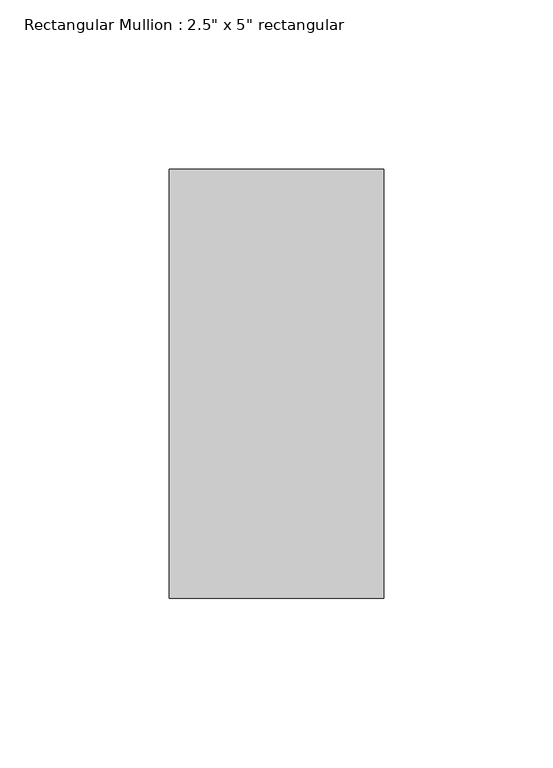
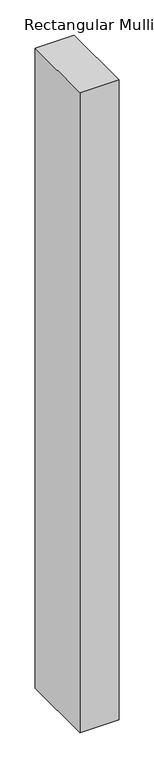
"""IFC4 building model written with IfcOpenShell, lengths in millimetres: member geometry."""

from ifc_helpers import new_model, si_unit, frame, origin, place, context, project, spatial, polyline, outline, extrude, source, transform, mapped, element, save


def member_766f1680(model_context):
    return source(origin(), model_context, "Body", "SweptSolid", [
        extrude(outline(polyline([(31.75, 63.5), (31.75, -63.5), (-31.75, -63.5), (-31.75, 63.5), (31.75, 63.5)])), frame((0.0, 0.0, -1104.8999998), z_axis=(0.0, 0.0, 1.0), x_axis=(1.0, 0.0, 0.0)), (0.0, 0.0, 1.0), 1104.8999998),
    ])


if __name__ == "__main__":
    model = new_model("IFC4")
    model_context = context("Model", 3, world=origin())
    ifc_project = project(units=[si_unit("LENGTHUNIT", "METRE", prefix="MILLI")], contexts=[model_context])
    site = spatial("IfcSite", under=ifc_project)
    building = spatial("IfcBuilding", under=site)
    placement = place(None, origin())
    member_shape = member_766f1680(model_context)
    element("IfcMember", 1, ObjectType="Rectangular Mullion : 2.5\" x 5\" rectangular", at=placement, inside=building, context=model_context, shape_type="MappedRepresentation", body=[
        mapped(member_shape, transform((0.0, 0.0, 0.0), x_axis=(1.0, 0.0, 0.0), y_axis=(0.0, 1.0, 0.0), z_axis=(0.0, 0.0, 1.0))),
    ])
    save(model, "model.ifc")

# Revit data of these elements
# Type "Rectangular Mullion : 2.5\" x 5\" rectangular"
#   built-in parameter 1007304 = 0.416667 (stored number, unit not read)
#   built-in parameter 1007301 = 0.104167 (stored number, unit not read)
#   built-in parameter 1007300 = 0.104167 (stored number, unit not read)
# Element 1 (IfcMember, "Rectangular Mullion : 2.5\" x 5\" rectangular")
#   Materials on its faces: "Aluminum"
# Materials
#   "Aluminum": class "Metal", colour RGB 247 247 247, transparency 0, Description = "Aluminum 6061", Cost = 0
